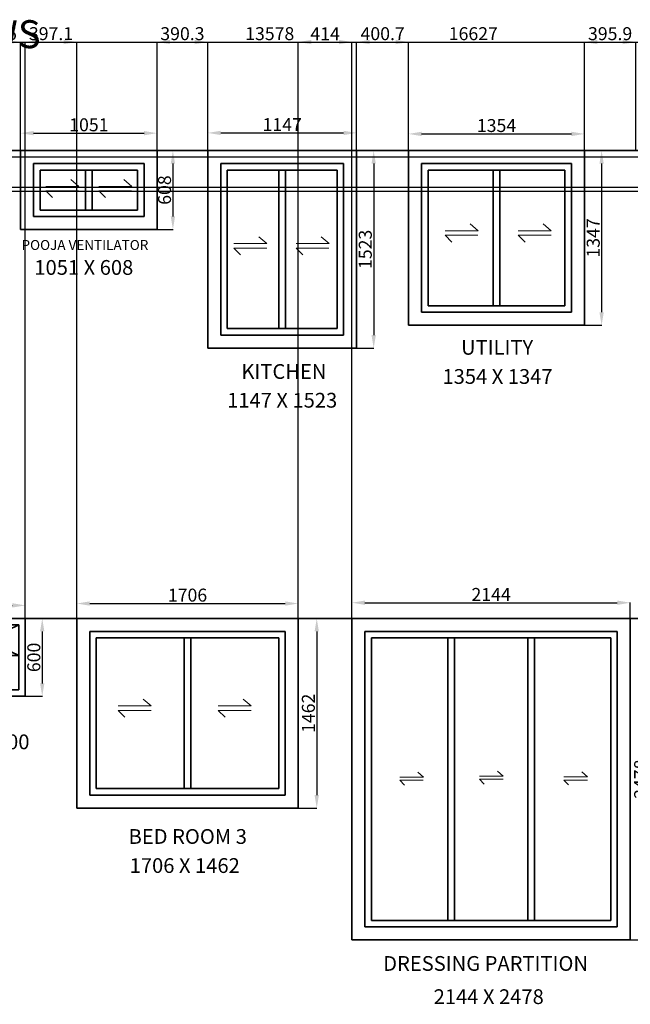
# Model space of a CAD drawing. Units: millimetres. Extents: x 5977 to 24120, y -1732 to 6209.
# Tile 2 of 3: x 11795 to 16498, y -1732 to 5862. Entities that reach past the tile are written whole.
import ezdxf

# ---------------------------------------------------------------- set-up
doc = ezdxf.new("R2010")
doc.units = ezdxf.units.MM
for name, color, linetype, lineweight in [('A-ANNO-DIMS', 2, 'Continuous', 18), ('A-ANNO-SYMB', 143, 'Continuous', 18), ('A-ANNO-TEXT', 7, 'Continuous', 25), ('A-GLAZ', 4, 'Continuous', 35)]:
    doc.layers.add(name, color=color, linetype=linetype, lineweight=lineweight)
doc.styles.get("Standard").update_dxf_attribs({"font": 'arial.ttf'})
doc.dimstyles.new('ISO-25', dxfattribs={"dimtxt": 100, "dimasz": 100, "dimexe": 1.25, "dimexo": 0.625, "dimtad": 1, "dimtxsty": 'Standard', "dimcen": 2.5, "dimadec": 0, "dimazin": 0, "dimtfac": 1, "dimtmove": 0, "dimatfit": 3, "dimfxl": 1, "dimarcsym": 0})

# ---------------------------------------------------------------- blocks, each defined once
blk = doc.blocks.new('*D5')
at = {"layer": 'A-ANNO-DIMS', "color": 0, "lineweight": -2, "transparency": 16777216}
for p, q in [((11802, 4852.8), (11802, 4988.1)), ((11902, 4986.9), (12753, 4986.9)), ((12853, 4852.8), (12853, 4988.1))]:
    blk.add_line(p, q, dxfattribs=at)
at = {"layer": 'A-ANNO-DIMS', "color": 0, "transparency": 16777216}
for points in [[(11902, 5003.5), (11902, 4970.2), (11802, 4986.9)], [(12753, 5003.5), (12753, 4970.2), (12853, 4986.9)]]:
    blk.add_solid(points, dxfattribs=at)
at = {"layer": 'Defpoints', "color": 0, "transparency": 16777216}
for p in [(12853, 4986.9), (11802, 4852.2), (12853, 4852.2)]:
    blk.add_point(p, dxfattribs=at)
at = {"layer": 'A-ANNO-DIMS', "color": 0, "transparency": 16777216, "insert": (12327.5, 5038.5), "char_height": 100, "attachment_point": 5}
blk.add_mtext('1051', dxfattribs=at)
blk = doc.blocks.new('*D6')
at = {"layer": 'A-ANNO-DIMS', "color": 0, "lineweight": -2, "transparency": 16777216}
for p, q in [((12853.6, 4852.2), (12976.1, 4852.2)), ((12974.8, 4752.2), (12974.8, 4344.2)), ((12853.6, 4244.2), (12976.1, 4244.2))]:
    blk.add_line(p, q, dxfattribs=at)
at = {"layer": 'A-ANNO-DIMS', "color": 0, "transparency": 16777216}
for points in [[(12958.2, 4752.2), (12991.5, 4752.2), (12974.8, 4852.2)], [(12958.2, 4344.2), (12991.5, 4344.2), (12974.8, 4244.2)]]:
    blk.add_solid(points, dxfattribs=at)
at = {"layer": 'Defpoints', "color": 0, "transparency": 16777216}
for p in [(12853, 4852.2), (12853, 4244.2), (12974.8, 4244.2)]:
    blk.add_point(p, dxfattribs=at)
at = {"layer": 'A-ANNO-DIMS', "color": 0, "transparency": 16777216, "insert": (12923.2, 4548.2), "char_height": 100, "attachment_point": 5, "rotation": 90}
blk.add_mtext('608', dxfattribs=at)
blk = doc.blocks.new('*D7')
at = {"layer": 'A-ANNO-DIMS', "color": 0, "lineweight": -2, "transparency": 16777216}
for p, q in [((13243.3, 4852.8), (13243.3, 4990.1)), ((13343.3, 4988.9), (14290.3, 4988.9)), ((14390.3, 4852.8), (14390.3, 4990.1))]:
    blk.add_line(p, q, dxfattribs=at)
at = {"layer": 'A-ANNO-DIMS', "color": 0, "transparency": 16777216}
for points in [[(13343.3, 5005.5), (13343.3, 4972.2), (13243.3, 4988.9)], [(14290.3, 5005.5), (14290.3, 4972.2), (14390.3, 4988.9)]]:
    blk.add_solid(points, dxfattribs=at)
at = {"layer": 'Defpoints', "color": 0, "transparency": 16777216}
for p in [(14390.3, 4988.9), (13243.3, 4852.2), (14390.3, 4852.2)]:
    blk.add_point(p, dxfattribs=at)
at = {"layer": 'A-ANNO-DIMS', "color": 0, "transparency": 16777216, "insert": (13816.8, 5039.7), "char_height": 100, "attachment_point": 5}
blk.add_mtext('1147', dxfattribs=at)
blk = doc.blocks.new('*D8')
at = {"layer": 'A-ANNO-DIMS', "color": 0, "lineweight": -2, "transparency": 16777216}
for p, q in [((14390.9, 4852.2), (14522.9, 4852.2)), ((14521.6, 4752.2), (14521.6, 3429.2)), ((14390.9, 3329.2), (14522.9, 3329.2))]:
    blk.add_line(p, q, dxfattribs=at)
at = {"layer": 'A-ANNO-DIMS', "color": 0, "transparency": 16777216}
for points in [[(14505, 4752.2), (14538.3, 4752.2), (14521.6, 4852.2)], [(14505, 3429.2), (14538.3, 3429.2), (14521.6, 3329.2)]]:
    blk.add_solid(points, dxfattribs=at)
at = {"layer": 'Defpoints', "color": 0, "transparency": 16777216}
for p in [(14390.3, 4852.2), (14390.3, 3329.2), (14521.6, 3329.2)]:
    blk.add_point(p, dxfattribs=at)
at = {"layer": 'A-ANNO-DIMS', "color": 0, "transparency": 16777216, "insert": (14469.9, 4090.7), "char_height": 100, "attachment_point": 5, "rotation": 90}
blk.add_mtext('1523', dxfattribs=at)
blk = doc.blocks.new('*D9')
at = {"layer": 'A-ANNO-DIMS', "color": 0, "lineweight": -2, "transparency": 16777216}
for p, q in [((14791, 4852.8), (14791, 4982.3)), ((14891, 4981.1), (16045, 4981.1)), ((16145, 4852.8), (16145, 4982.3))]:
    blk.add_line(p, q, dxfattribs=at)
at = {"layer": 'A-ANNO-DIMS', "color": 0, "transparency": 16777216}
for points in [[(14891, 4997.8), (14891, 4964.4), (14791, 4981.1)], [(16045, 4997.8), (16045, 4964.4), (16145, 4981.1)]]:
    blk.add_solid(points, dxfattribs=at)
at = {"layer": 'Defpoints', "color": 0, "transparency": 16777216}
for p in [(16145, 4981.1), (14791, 4852.2), (16145, 4852.2)]:
    blk.add_point(p, dxfattribs=at)
at = {"layer": 'A-ANNO-DIMS', "color": 0, "transparency": 16777216, "insert": (15468, 5032.8), "char_height": 100, "attachment_point": 5}
blk.add_mtext('1354', dxfattribs=at)
blk = doc.blocks.new('*D10')
at = {"layer": 'A-ANNO-DIMS', "color": 0, "lineweight": -2, "transparency": 16777216}
for p, q in [((16145.6, 4852.2), (16278.9, 4852.2)), ((16277.6, 4752.2), (16277.6, 3605.2)), ((16145.6, 3505.2), (16278.9, 3505.2))]:
    blk.add_line(p, q, dxfattribs=at)
at = {"layer": 'A-ANNO-DIMS', "color": 0, "transparency": 16777216}
for points in [[(16260.9, 4752.2), (16294.3, 4752.2), (16277.6, 4852.2)], [(16260.9, 3605.2), (16294.3, 3605.2), (16277.6, 3505.2)]]:
    blk.add_solid(points, dxfattribs=at)
at = {"layer": 'Defpoints', "color": 0, "transparency": 16777216}
for p in [(16145, 4852.2), (16145, 3505.2), (16277.6, 3505.2)]:
    blk.add_point(p, dxfattribs=at)
at = {"layer": 'A-ANNO-DIMS', "color": 0, "transparency": 16777216, "insert": (16225.9, 4178.7), "char_height": 100, "attachment_point": 5, "rotation": 90}
blk.add_mtext('1347', dxfattribs=at)
blk = doc.blocks.new('*D27')
at = {"layer": 'A-ANNO-DIMS', "color": 0, "lineweight": -2, "transparency": 16777216}
for p, q in [((11237.4, 1244.3), (11237.4, 1346.1)), ((11337.4, 1344.9), (11737.4, 1344.9)), ((11837.4, 1244.3), (11837.4, 1346.1))]:
    blk.add_line(p, q, dxfattribs=at)
at = {"layer": 'A-ANNO-DIMS', "color": 0, "transparency": 16777216}
for points in [[(11337.4, 1361.5), (11337.4, 1328.2), (11237.4, 1344.9)], [(11737.4, 1361.5), (11737.4, 1328.2), (11837.4, 1344.9)]]:
    blk.add_solid(points, dxfattribs=at)
at = {"layer": 'Defpoints', "color": 0, "transparency": 16777216}
for p in [(11837.4, 1344.9), (11237.4, 1243.7), (11837.4, 1243.7)]:
    blk.add_point(p, dxfattribs=at)
at = {"layer": 'A-ANNO-DIMS', "color": 0, "transparency": 16777216, "insert": (11537.4, 1396.6), "char_height": 100, "attachment_point": 5}
blk.add_mtext('600', dxfattribs=at)
blk = doc.blocks.new('*D28')
at = {"layer": 'A-ANNO-DIMS', "color": 0, "lineweight": -2, "transparency": 16777216}
for p, q in [((11838, 1243.7), (11969.4, 1243.7)), ((11968.1, 1143.7), (11968.1, 743.7)), ((11838, 643.7), (11969.4, 643.7))]:
    blk.add_line(p, q, dxfattribs=at)
at = {"layer": 'A-ANNO-DIMS', "color": 0, "transparency": 16777216}
for points in [[(11951.4, 1143.7), (11984.8, 1143.7), (11968.1, 1243.7)], [(11951.4, 743.7), (11984.8, 743.7), (11968.1, 643.7)]]:
    blk.add_solid(points, dxfattribs=at)
at = {"layer": 'Defpoints', "color": 0, "transparency": 16777216}
for p in [(11837.4, 1243.7), (11837.4, 643.7), (11968.1, 643.7)]:
    blk.add_point(p, dxfattribs=at)
at = {"layer": 'A-ANNO-DIMS', "color": 0, "transparency": 16777216, "insert": (11916.4, 943.7), "char_height": 100, "attachment_point": 5, "rotation": 90}
blk.add_mtext('600', dxfattribs=at)
blk = doc.blocks.new('*D29')
at = {"layer": 'A-ANNO-DIMS', "color": 0, "lineweight": -2, "transparency": 16777216}
for p, q in [((12234.5, 1244.3), (12234.5, 1360.6)), ((12334.5, 1359.4), (13840.5, 1359.4)), ((13940.5, 1244.3), (13940.5, 1360.6))]:
    blk.add_line(p, q, dxfattribs=at)
at = {"layer": 'A-ANNO-DIMS', "color": 0, "transparency": 16777216}
for points in [[(12334.5, 1376), (12334.5, 1342.7), (12234.5, 1359.4)], [(13840.5, 1376), (13840.5, 1342.7), (13940.5, 1359.4)]]:
    blk.add_solid(points, dxfattribs=at)
at = {"layer": 'Defpoints', "color": 0, "transparency": 16777216}
for p in [(13940.5, 1359.4), (12234.5, 1243.7), (13940.5, 1243.7)]:
    blk.add_point(p, dxfattribs=at)
at = {"layer": 'A-ANNO-DIMS', "color": 0, "transparency": 16777216, "insert": (13087.5, 1411.1), "char_height": 100, "attachment_point": 5}
blk.add_mtext('1706', dxfattribs=at)
blk = doc.blocks.new('*D30')
at = {"layer": 'A-ANNO-DIMS', "color": 0, "lineweight": -2, "transparency": 16777216}
for p, q in [((13941.1, 1243.7), (14084.3, 1243.7)), ((14083.1, 1143.7), (14083.1, -118.3)), ((13941.1, -218.3), (14084.3, -218.3))]:
    blk.add_line(p, q, dxfattribs=at)
at = {"layer": 'A-ANNO-DIMS', "color": 0, "transparency": 16777216}
for points in [[(14066.4, 1143.7), (14099.7, 1143.7), (14083.1, 1243.7)], [(14066.4, -118.3), (14099.7, -118.3), (14083.1, -218.3)]]:
    blk.add_solid(points, dxfattribs=at)
at = {"layer": 'Defpoints', "color": 0, "transparency": 16777216}
for p in [(13940.5, 1243.7), (13940.5, -218.3), (14083.1, -218.3)]:
    blk.add_point(p, dxfattribs=at)
at = {"layer": 'A-ANNO-DIMS', "color": 0, "transparency": 16777216, "insert": (14031.4, 512.7), "char_height": 100, "attachment_point": 5, "rotation": 90}
blk.add_mtext('1462', dxfattribs=at)
blk = doc.blocks.new('*D31')
at = {"layer": 'A-ANNO-DIMS', "color": 0, "lineweight": -2, "transparency": 16777216}
for p, q in [((14354.5, 1244.3), (14354.5, 1366.7)), ((14454.5, 1365.4), (16398.5, 1365.4)), ((16498.5, 1244.3), (16498.5, 1366.7))]:
    blk.add_line(p, q, dxfattribs=at)
at = {"layer": 'A-ANNO-DIMS', "color": 0, "transparency": 16777216}
for points in [[(14454.5, 1382.1), (14454.5, 1348.8), (14354.5, 1365.4)], [(16398.5, 1382.1), (16398.5, 1348.8), (16498.5, 1365.4)]]:
    blk.add_solid(points, dxfattribs=at)
at = {"layer": 'Defpoints', "color": 0, "transparency": 16777216}
for p in [(16498.5, 1365.4), (14354.5, 1243.7), (16498.5, 1243.7)]:
    blk.add_point(p, dxfattribs=at)
at = {"layer": 'A-ANNO-DIMS', "color": 0, "transparency": 16777216, "insert": (15426.5, 1416.3), "char_height": 100, "attachment_point": 5}
blk.add_mtext('2144', dxfattribs=at)
blk = doc.blocks.new('*D32')
at = {"layer": 'A-ANNO-DIMS', "color": 0, "lineweight": -2, "transparency": 16777216}
for p, q in [((16499.1, 1243.7), (16644.2, 1243.7)), ((16643, 1143.7), (16643, -1134.3)), ((16499.1, -1234.3), (16644.2, -1234.3))]:
    blk.add_line(p, q, dxfattribs=at)
at = {"layer": 'A-ANNO-DIMS', "color": 0, "transparency": 16777216}
for points in [[(16626.3, 1143.7), (16659.6, 1143.7), (16643, 1243.7)], [(16626.3, -1134.3), (16659.6, -1134.3), (16643, -1234.3)]]:
    blk.add_solid(points, dxfattribs=at)
at = {"layer": 'Defpoints', "color": 0, "transparency": 16777216}
for p in [(16498.5, 1243.7), (16498.5, -1234.3), (16643, -1234.3)]:
    blk.add_point(p, dxfattribs=at)
at = {"layer": 'A-ANNO-DIMS', "color": 0, "transparency": 16777216, "insert": (16591.3, 4.7), "char_height": 100, "attachment_point": 5, "rotation": 90}
blk.add_mtext('2478', dxfattribs=at)
blk = doc.blocks.new('WIN-600x600-TOILET')
for p, q in [((16540.9, 4852.2), (16540.9, 4252.2)), ((16590.9, 4802.2), (16590.9, 4302.2)), ((16590.9, 4802.2), (17090.9, 4802.2)), ((16590.9, 4567.2), (17090.9, 4802.2)), ((17090.9, 4567.2), (16590.9, 4802.2)), ((17090.9, 4302.2), (17090.9, 4802.2)), ((17140.9, 4252.2), (17140.9, 4852.2)), ((16590.9, 4567.2), (17090.9, 4567.2)), ((16590.9, 4302.2), (17090.9, 4302.2)), ((16540.9, 4252.2), (17140.9, 4252.2))]:
    blk.add_line(p, q)
blk = doc.blocks.new('ARROW-SLIDE')
for p, q in [((14721.8, 21.3), (14904.6, 21.3)), ((14904.6, 21.3), (14860.5, 58.6)), ((14721.8, -3.8), (14904.1, -3.8)), ((14721.8, -3.8), (14759.4, -41.4))]:
    blk.add_line(p, q)
blk = doc.blocks.new('ARROW-SLIDE-LG')
for p, q in [((7575.1, 4322.2), (7513.8, 4374)), ((7321, 4287.2), (7574.5, 4287.2)), ((7321, 4287.2), (7373.4, 4234.9)), ((7321.1, 4322.2), (7575.1, 4322.2))]:
    blk.add_line(p, q)
blk = doc.blocks.new('*D41')
at = {"layer": 'A-ANNO-DIMS', "color": 0, "lineweight": -2, "transparency": 16777216}
for p, q in [((6975.8, 4852.8), (6975.8, 5690.9)), ((7075.8, 5689.7), (23502.6, 5689.7)), ((23602.6, 4852.8), (23602.6, 5690.9))]:
    blk.add_line(p, q, dxfattribs=at)
at = {"layer": 'A-ANNO-DIMS', "color": 0, "transparency": 16777216}
for points in [[(7075.8, 5706.3), (7075.8, 5673), (6975.8, 5689.7)], [(23502.6, 5706.3), (23502.6, 5673), (23602.6, 5689.7)]]:
    blk.add_solid(points, dxfattribs=at)
at = {"layer": 'Defpoints', "color": 0, "transparency": 16777216}
for p in [(23602.6, 5689.7), (6975.8, 4852.2), (23602.6, 4852.2)]:
    blk.add_point(p, dxfattribs=at)
at = {"layer": 'A-ANNO-DIMS', "color": 0, "transparency": 16777216, "insert": (15289.2, 5741.3), "char_height": 100, "attachment_point": 5}
blk.add_mtext('16627', dxfattribs=at)
blk = doc.blocks.new('*D42')
at = {"layer": 'A-ANNO-DIMS', "color": 0, "lineweight": -2, "transparency": 16777216}
for p, q in [((6931.9, 1244.3), (6931.9, 5690.9)), ((7031.9, 5689.7), (20409.7, 5689.7)), ((20509.7, 1244.3), (20509.7, 5690.9))]:
    blk.add_line(p, q, dxfattribs=at)
at = {"layer": 'A-ANNO-DIMS', "color": 0, "transparency": 16777216}
for points in [[(7031.9, 5706.3), (7031.9, 5673), (6931.9, 5689.7)], [(20409.7, 5706.3), (20409.7, 5673), (20509.7, 5689.7)]]:
    blk.add_solid(points, dxfattribs=at)
at = {"layer": 'Defpoints', "color": 0, "transparency": 16777216}
for p in [(20509.7, 5689.7), (6931.9, 1243.7), (20509.7, 1243.7)]:
    blk.add_point(p, dxfattribs=at)
at = {"layer": 'A-ANNO-DIMS', "color": 0, "transparency": 16777216, "insert": (13720.8, 5741.4), "char_height": 100, "attachment_point": 5}
blk.add_mtext('13578', dxfattribs=at)
blk = doc.blocks.new('*D45')
at = {"layer": 'A-ANNO-DIMS', "color": 0, "lineweight": -2, "transparency": 16777216}
for p, q in [((11404.5, 4852.8), (11404.5, 5690.9)), ((11504.5, 5689.7), (11702, 5689.7)), ((11802, 4852.8), (11802, 5690.9))]:
    blk.add_line(p, q, dxfattribs=at)
at = {"layer": 'A-ANNO-DIMS', "color": 0, "transparency": 16777216}
for points in [[(11504.5, 5706.3), (11504.5, 5673), (11404.5, 5689.7)], [(11702, 5706.3), (11702, 5673), (11802, 5689.7)]]:
    blk.add_solid(points, dxfattribs=at)
at = {"layer": 'Defpoints', "color": 0, "transparency": 16777216}
for p in [(11802, 5689.7), (11404.5, 4852.2), (11802, 4852.2)]:
    blk.add_point(p, dxfattribs=at)
at = {"layer": 'A-ANNO-DIMS', "color": 0, "transparency": 16777216, "insert": (11603.2, 5741.4), "char_height": 100, "attachment_point": 5}
blk.add_mtext('397.5', dxfattribs=at)
blk = doc.blocks.new('*D46')
at = {"layer": 'A-ANNO-DIMS', "color": 0, "lineweight": -2, "transparency": 16777216}
for p, q in [((12853, 4852.8), (12853, 5690.9)), ((12953, 5689.7), (13143.3, 5689.7)), ((13243.3, 4852.8), (13243.3, 5690.9))]:
    blk.add_line(p, q, dxfattribs=at)
at = {"layer": 'A-ANNO-DIMS', "color": 0, "transparency": 16777216}
for points in [[(12953, 5706.3), (12953, 5673), (12853, 5689.7)], [(13143.3, 5706.3), (13143.3, 5673), (13243.3, 5689.7)]]:
    blk.add_solid(points, dxfattribs=at)
at = {"layer": 'Defpoints', "color": 0, "transparency": 16777216}
for p in [(13243.3, 5689.7), (12853, 4852.2), (13243.3, 4852.2)]:
    blk.add_point(p, dxfattribs=at)
at = {"layer": 'A-ANNO-DIMS', "color": 0, "transparency": 16777216, "insert": (13048.1, 5741.4), "char_height": 100, "attachment_point": 5}
blk.add_mtext('390.3', dxfattribs=at)
blk = doc.blocks.new('*D47')
at = {"layer": 'A-ANNO-DIMS', "color": 0, "lineweight": -2, "transparency": 16777216}
for p, q in [((14390.3, 4852.8), (14390.3, 5690.9)), ((14490.3, 5689.7), (14691, 5689.7)), ((14791, 4852.8), (14791, 5690.9))]:
    blk.add_line(p, q, dxfattribs=at)
at = {"layer": 'A-ANNO-DIMS', "color": 0, "transparency": 16777216}
for points in [[(14490.3, 5706.3), (14490.3, 5673), (14390.3, 5689.7)], [(14691, 5706.3), (14691, 5673), (14791, 5689.7)]]:
    blk.add_solid(points, dxfattribs=at)
at = {"layer": 'Defpoints', "color": 0, "transparency": 16777216}
for p in [(14791, 5689.7), (14390.3, 4852.2), (14791, 4852.2)]:
    blk.add_point(p, dxfattribs=at)
at = {"layer": 'A-ANNO-DIMS', "color": 0, "transparency": 16777216, "insert": (14590.7, 5741.3), "char_height": 100, "attachment_point": 5}
blk.add_mtext('400.7', dxfattribs=at)
blk = doc.blocks.new('*D48')
at = {"layer": 'A-ANNO-DIMS', "color": 0, "lineweight": -2, "transparency": 16777216}
for p, q in [((16145, 4852.8), (16145, 5690.9)), ((16245, 5689.7), (16440.9, 5689.7)), ((16540.9, 4852.8), (16540.9, 5690.9))]:
    blk.add_line(p, q, dxfattribs=at)
at = {"layer": 'A-ANNO-DIMS', "color": 0, "transparency": 16777216}
for points in [[(16245, 5706.3), (16245, 5673), (16145, 5689.7)], [(16440.9, 5706.3), (16440.9, 5673), (16540.9, 5689.7)]]:
    blk.add_solid(points, dxfattribs=at)
at = {"layer": 'Defpoints', "color": 0, "transparency": 16777216}
for p in [(16540.9, 5689.7), (16145, 4852.2), (16540.9, 4852.2)]:
    blk.add_point(p, dxfattribs=at)
at = {"layer": 'A-ANNO-DIMS', "color": 0, "transparency": 16777216, "insert": (16343, 5741.4), "char_height": 100, "attachment_point": 5}
blk.add_mtext('395.9', dxfattribs=at)
blk = doc.blocks.new('*D55')
at = {"layer": 'A-ANNO-DIMS', "color": 0, "lineweight": -2, "transparency": 16777216}
for p, q in [((11837.4, 1244.3), (11837.4, 5690.9)), ((11937.4, 5689.7), (12134.5, 5689.7)), ((12234.5, 1244.3), (12234.5, 5690.9))]:
    blk.add_line(p, q, dxfattribs=at)
at = {"layer": 'A-ANNO-DIMS', "color": 0, "transparency": 16777216}
for points in [[(11937.4, 5706.3), (11937.4, 5673), (11837.4, 5689.7)], [(12134.5, 5706.3), (12134.5, 5673), (12234.5, 5689.7)]]:
    blk.add_solid(points, dxfattribs=at)
at = {"layer": 'Defpoints', "color": 0, "transparency": 16777216}
for p in [(12234.5, 5689.7), (11837.4, 1243.7), (12234.5, 1243.7)]:
    blk.add_point(p, dxfattribs=at)
at = {"layer": 'A-ANNO-DIMS', "color": 0, "transparency": 16777216, "insert": (12035.9, 5741.4), "char_height": 100, "attachment_point": 5}
blk.add_mtext('397.1', dxfattribs=at)
blk = doc.blocks.new('*D56')
at = {"layer": 'A-ANNO-DIMS', "color": 0, "lineweight": -2, "transparency": 16777216}
for p, q in [((13940.5, 1244.3), (13940.5, 5690.9)), ((14040.5, 5689.7), (14254.5, 5689.7)), ((14354.5, 1244.3), (14354.5, 5690.9))]:
    blk.add_line(p, q, dxfattribs=at)
at = {"layer": 'A-ANNO-DIMS', "color": 0, "transparency": 16777216}
for points in [[(14040.5, 5706.3), (14040.5, 5673), (13940.5, 5689.7)], [(14254.5, 5706.3), (14254.5, 5673), (14354.5, 5689.7)]]:
    blk.add_solid(points, dxfattribs=at)
at = {"layer": 'Defpoints', "color": 0, "transparency": 16777216}
for p in [(14354.5, 5689.7), (13940.5, 1243.7), (14354.5, 1243.7)]:
    blk.add_point(p, dxfattribs=at)
at = {"layer": 'A-ANNO-DIMS', "color": 0, "transparency": 16777216, "insert": (14147.5, 5740.5), "char_height": 100, "attachment_point": 5}
blk.add_mtext('414', dxfattribs=at)
blk = doc.blocks.new('*D67')
at = {"layer": 'A-ANNO-DIMS', "color": 0, "lineweight": -2, "transparency": 16777216}
for p, q in [((16590.3, 4802.2), (6093.2, 4802.2)), ((6094.4, 4702.2), (6094.4, 4667.2)), ((16590.3, 4567.2), (6093.2, 4567.2))]:
    blk.add_line(p, q, dxfattribs=at)
at = {"layer": 'A-ANNO-DIMS', "color": 0, "transparency": 16777216}
for points in [[(6077.8, 4702.2), (6111.1, 4702.2), (6094.4, 4802.2)], [(6077.8, 4667.2), (6111.1, 4667.2), (6094.4, 4567.2)]]:
    blk.add_solid(points, dxfattribs=at)
at = {"layer": 'Defpoints', "color": 0, "transparency": 16777216}
for p in [(16590.9, 4802.2), (6094.4, 4567.2), (16590.9, 4567.2)]:
    blk.add_point(p, dxfattribs=at)
at = {"layer": 'A-ANNO-DIMS', "color": 0, "transparency": 16777216, "insert": (6042.7, 4684.7), "char_height": 100, "attachment_point": 5, "rotation": 90}
blk.add_mtext('235', dxfattribs=at)
blk = doc.blocks.new('*D68')
at = {"layer": 'A-ANNO-DIMS', "color": 0, "lineweight": -2, "transparency": 16777216}
for p, q in [((6094.4, 4667.2), (6094.4, 4767.2)), ((16590.3, 4567.2), (6093.2, 4567.2)), ((6094.4, 4567.2), (6094.4, 4537.2)), ((16590.3, 4537.2), (6093.2, 4537.2)), ((6094.4, 4437.2), (6094.4, 4193.1))]:
    blk.add_line(p, q, dxfattribs=at)
at = {"layer": 'A-ANNO-DIMS', "color": 0, "transparency": 16777216}
for points in [[(6077.8, 4667.2), (6111.1, 4667.2), (6094.4, 4567.2)], [(6077.8, 4437.2), (6111.1, 4437.2), (6094.4, 4537.2)]]:
    blk.add_solid(points, dxfattribs=at)
at = {"layer": 'Defpoints', "color": 0, "transparency": 16777216}
for p in [(16590.9, 4567.2), (6094.4, 4537.2), (16590.9, 4537.2)]:
    blk.add_point(p, dxfattribs=at)
at = {"layer": 'A-ANNO-DIMS', "color": 0, "transparency": 16777216, "insert": (6042.7, 4265.1), "char_height": 100, "attachment_point": 5, "rotation": 90}
blk.add_mtext('30', dxfattribs=at)

msp = doc.modelspace()

# ---------------------------------------------------------------- linework, layer by layer
at = {"layer": 'A-GLAZ'}
for p, q in [((6975.757, 4852.16), (19747.827, 4852.16)), ((11801.995, 4852.16), (11801.995, 4244.16)), ((12852.995, 4244.16), (12852.995, 4852.16)), ((13243.287, 4852.16), (13243.287, 3329.16)), ((14390.287, 3329.16), (14390.287, 4852.16)), ((14791.025, 4852.16), (14791.025, 3505.16)), ((16145.025, 3505.16), (16145.025, 4852.16)), ((11901.995, 4752.16), (12752.995, 4752.16)), ((11901.995, 4752.16), (11901.995, 4344.16)), ((12752.995, 4344.16), (12752.995, 4752.16)), ((13343.287, 4752.16), (13343.287, 3429.16)), ((13343.287, 4752.16), (14290.287, 4752.16)), ((14290.287, 3429.16), (14290.287, 4752.16)), ((14891.025, 4752.16), (16045.025, 4752.16)), ((14891.025, 4752.16), (14891.025, 3605.16)), ((16045.025, 3605.16), (16045.025, 4752.16)), ((11951.995, 4702.16), (12702.995, 4702.16)), ((11951.995, 4702.16), (11951.995, 4394.16)), ((12302.495, 4702.16), (12302.495, 4394.16)), ((12352.495, 4702.16), (12352.495, 4394.16)), ((12702.995, 4394.16), (12702.995, 4702.16)), ((13393.287, 4702.16), (13393.287, 3479.16)), ((13393.287, 4702.16), (14240.287, 4702.16)), ((13791.787, 3479.16), (13791.787, 4702.16)), ((13841.787, 3479.16), (13841.787, 4702.16)), ((14240.287, 3479.16), (14240.287, 4702.16)), ((14941.025, 4702.16), (15995.025, 4702.16)), ((14941.025, 4702.16), (14941.025, 3655.16)), ((15443.025, 4702.16), (15443.025, 3655.16)), ((15493.025, 4702.16), (15493.025, 3655.16)), ((15995.025, 3655.16), (15995.025, 4702.16)), ((11901.995, 4344.16), (12752.995, 4344.16)), ((11951.995, 4394.16), (12702.995, 4394.16)), ((11801.995, 4244.16), (12852.995, 4244.16)), ((14941.025, 3655.16), (15995.025, 3655.16)), ((14891.025, 3605.16), (16045.025, 3605.16)), ((14791.025, 3505.16), (16145.025, 3505.16)), ((13343.287, 3429.16), (14290.287, 3429.16)), ((13393.287, 3479.16), (14240.287, 3479.16)), ((13243.287, 3329.16), (14390.287, 3329.16)), ((6931.935, 1243.651), (20509.687, 1243.651)), ((12234.489, 1243.651), (12234.489, -218.349)), ((13940.489, -218.349), (13940.489, 1243.651)), ((14354.47, 1243.651), (14354.47, -1234.349)), ((16498.47, -1234.349), (16498.47, 1243.651)), ((12334.489, 1143.651), (13840.489, 1143.651)), ((12334.489, 1143.651), (12334.489, -118.349)), ((13840.489, -118.349), (13840.489, 1143.651)), ((14454.47, 1143.651), (16398.47, 1143.651)), ((14454.47, 1143.651), (14454.47, -1134.349)), ((16398.47, -1134.349), (16398.47, 1143.651)), ((12384.489, 1093.651), (13790.489, 1093.651)), ((12384.489, 1093.651), (12384.489, -68.349)), ((13062.489, -68.349), (13062.489, 1093.651)), ((13112.489, -68.349), (13112.489, 1093.651)), ((13790.489, -68.349), (13790.489, 1093.651)), ((14504.47, 1093.651), (16348.47, 1093.651)), ((14504.47, 1093.651), (14504.47, -1084.349)), ((15093.47, 1093.651), (15093.47, -1084.349)), ((15143.47, 1093.651), (15143.47, -1084.349)), ((15709.47, -1084.349), (15709.47, 1093.651)), ((15759.47, -1084.349), (15759.47, 1093.651)), ((16348.47, -1084.349), (16348.47, 1093.651)), ((12384.489, -68.349), (13790.489, -68.349)), ((12334.489, -118.349), (13840.489, -118.349)), ((12234.489, -218.349), (13940.489, -218.349)), ((14454.47, -1134.349), (16398.47, -1134.349)), ((14504.47, -1084.349), (16348.47, -1084.349)), ((14354.47, -1234.349), (16498.47, -1234.349))]:
    msp.add_line(p, q, dxfattribs=at)

# ---------------------------------------------------------------- block references
at = {"layer": 'A-ANNO-SYMB'}
for name, p in [('ARROW-SLIDE-LG', (4674.265, 254.552)), ('ARROW-SLIDE-LG', (5082.199, 254.552)), ('ARROW-SLIDE-LG', (7750.759, -87.584)), ('ARROW-SLIDE-LG', (8313.981, -87.584)), ('ARROW-SLIDE-LG', (6122.827, -186.478)), ('ARROW-SLIDE-LG', (6602.723, -186.478)), ('ARROW-SLIDE-LG', (5231.795, -3751.741)), ('ARROW-SLIDE-LG', (6003.076, -3751.741)), ('ARROW-SLIDE', (0, 0)), ('ARROW-SLIDE', (613.878, 7.209)), ('ARROW-SLIDE', (1264.06, 1.512))]:
    msp.add_blockref(name, p, dxfattribs=at)
at = {"layer": 'A-GLAZ'}
msp.add_blockref('WIN-600x600-TOILET', (-5303.553, -3608.51), dxfattribs=at)

# ---------------------------------------------------------------- texts
at = {"layer": 'A-ANNO-TEXT'}
for s, height, p in [('1ST,2ND AND 3RD FLOOR WINDOWS', 215.75319, (7010.9, 5642.477)), ('POOJA VENTILATOR', 76.2677, (11808.62, 4086.344)), ('1051 X 608', 113.8754, (11907.482, 3894.342)), ('UTILITY', 113.8754, (15194.569, 3278.29)), ('KITCHEN', 113.8754, (13502.564, 3091.776)), ('1354 X 1347', 113.87539, (15051.425, 3053.397)), ('1147 X 1523', 113.87539, (13392.348, 2870.088)), ('600 X 600', 113.8754, (11193.932, 235.504)), ('BED ROOM 3', 113.8754, (12633.361, -494.292)), ('1706 X 1462', 113.87539, (12641.836, -718.497)), ('DRESSING PARTITION', 113.87539, (14594.667, -1473.647)), ('2144 X 2478', 113.87539, (14983.725, -1729.682))]:
    msp.add_text(s, height=height, dxfattribs=at).set_placement(p)

# ---------------------------------------------------------------- dimensions: what is measured, and where the dimension line sits
at = {"layer": 'A-ANNO-DIMS'}
for base, p1, p2, override, picture, middle in [((20509.687, 5689.66), (6931.935, 1243.651), (20509.687, 1243.651), {"dimdec": 0, "dimlfac": 1, "dimrnd": 0, "dimzin": 0, "dimdsep": 46, "dimlunit": 2}, '*D42', (13720.811, 5741.377)), ((23602.612, 5689.66), (6975.757, 4852.16), (23602.612, 4852.16), {"dimdec": 0, "dimlfac": 1, "dimrnd": 0, "dimzin": 0, "dimdsep": 46, "dimlunit": 2}, '*D41', (15289.184, 5741.343)), ((11801.995, 5689.66), (11404.482, 4852.16), (11801.995, 4852.16), {"dimdec": 1, "dimlfac": 1, "dimrnd": 0, "dimzin": 0, "dimdsep": 46, "dimlunit": 2}, '*D45', (11603.238, 5741.377)), ((12234.489, 5689.66), (11837.351, 1243.651), (12234.489, 1243.651), {"dimdec": 1, "dimlfac": 1, "dimrnd": 0, "dimzin": 0, "dimdsep": 46, "dimlunit": 2}, '*D55', (12035.92, 5741.377)), ((13243.287, 5689.66), (12852.995, 4852.16), (13243.287, 4852.16), {"dimdec": 1, "dimlfac": 1, "dimrnd": 0, "dimzin": 0, "dimdsep": 46, "dimlunit": 2}, '*D46', (13048.141, 5741.377)), ((14354.47, 5689.66), (13940.489, 1243.651), (14354.47, 1243.651), {"dimdec": 0, "dimlfac": 1, "dimrnd": 0, "dimzin": 0, "dimdsep": 46, "dimlunit": 2}, '*D56', (14147.48, 5740.49)), ((14791.025, 5689.66), (14390.287, 4852.16), (14791.025, 4852.16), {"dimdec": 1, "dimlfac": 1, "dimrnd": 0, "dimzin": 0, "dimdsep": 46, "dimlunit": 2}, '*D47', (14590.656, 5741.343)), ((16540.904, 5689.66), (16145.025, 4852.16), (16540.904, 4852.16), {"dimdec": 1, "dimlfac": 1, "dimrnd": 0, "dimzin": 0, "dimdsep": 46, "dimlunit": 2}, '*D48', (16342.964, 5741.377)), ((12852.995, 4986.864), (11801.995, 4852.16), (12852.995, 4852.16), {"dimclrd": 0, "dimclre": 0, "dimclrt": 0}, '*D5', (12327.495, 5038.546)), ((14390.287, 4988.851), (13243.287, 4852.16), (14390.287, 4852.16), {"dimclrd": 0, "dimclre": 0, "dimclrt": 0}, '*D7', (13816.787, 5039.681)), ((16145.025, 4981.088), (14791.025, 4852.16), (16145.025, 4852.16), {"dimclrd": 0, "dimclre": 0, "dimclrt": 0}, '*D9', (15468.025, 5032.804)), ((11837.351, 1344.88), (11237.351, 1243.651), (11837.351, 1243.651), {"dimclrd": 0, "dimclre": 0, "dimclrt": 0}, '*D27', (11537.351, 1396.562)), ((13940.489, 1359.371), (12234.489, 1243.651), (13940.489, 1243.651), {"dimclrd": 0, "dimclre": 0, "dimclrt": 0}, '*D29', (13087.489, 1411.054)), ((16498.47, 1365.437), (14354.47, 1243.651), (16498.47, 1243.651), {"dimclrd": 0, "dimclre": 0, "dimclrt": 0}, '*D31', (15426.47, 1416.267))]:
    dim = msp.add_linear_dim(base=base, p1=p1, p2=p2, dimstyle='ISO-25', override=override, dxfattribs=at)
    dim.commit()
    dim.dimension.update_dxf_attribs({"geometry": picture, "text_midpoint": middle})
for base, p1, p2, override, picture, middle in [((6094.435, 4567.16), (16590.904, 4802.16), (16590.904, 4567.16), {"dimdec": 0, "dimlfac": 1, "dimrnd": 0, "dimzin": 0, "dimdsep": 46, "dimlunit": 2}, '*D67', (6042.718, 4684.66)), ((12974.846, 4244.16), (12852.995, 4852.16), (12852.995, 4244.16), {"dimclrd": 0, "dimclre": 0, "dimclrt": 0}, '*D6', (12923.164, 4548.16)), ((14521.637, 3329.16), (14390.287, 4852.16), (14390.287, 3329.16), {"dimclrd": 0, "dimclre": 0, "dimclrt": 0}, '*D8', (14469.921, 4090.66)), ((16277.606, 3505.16), (16145.025, 4852.16), (16145.025, 3505.16), {"dimclrd": 0, "dimclre": 0, "dimclrt": 0}, '*D10', (16225.89, 4178.66)), ((6094.435, 4537.16), (16590.904, 4567.16), (16590.904, 4537.16), {"dimdec": 0, "dimlfac": 1, "dimrnd": 0, "dimzin": 0, "dimdsep": 46, "dimlunit": 2}, '*D68', (6042.718, 4265.117)), ((11968.112, 643.651), (11837.351, 1243.651), (11837.351, 643.651), {"dimclrd": 0, "dimclre": 0, "dimclrt": 0}, '*D28', (11916.429, 943.651)), ((14083.064, -218.349), (13940.489, 1243.651), (13940.489, -218.349), {"dimclrd": 0, "dimclre": 0, "dimclrt": 0}, '*D30', (14031.382, 512.651)), ((16642.963, -1234.349), (16498.47, 1243.651), (16498.47, -1234.349), {"dimclrd": 0, "dimclre": 0, "dimclrt": 0}, '*D32', (16591.281, 4.651))]:
    dim = msp.add_linear_dim(base=base, p1=p1, p2=p2, angle=90, dimstyle='ISO-25', override=override, dxfattribs=at)
    dim.commit()
    dim.dimension.update_dxf_attribs({"geometry": picture, "text_midpoint": middle})

doc.saveas('drawing.dxf')
